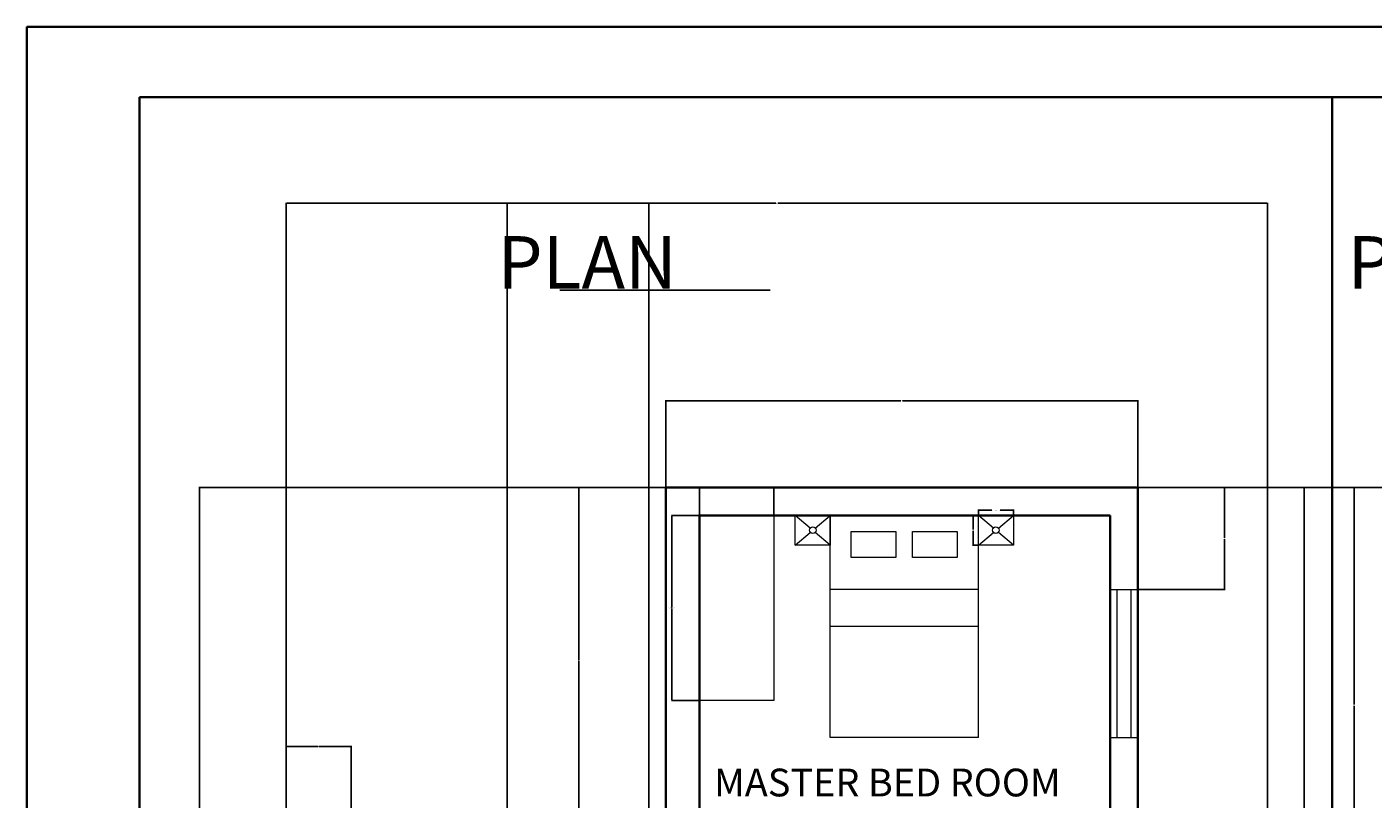
# Model space of a CAD drawing. Units: inches. Extents: x 1762 to 3150, y 1680 to 2382.
# Tile 4 of 6: x 1762 to 2199, y 2132 to 2382. Entities that reach past the tile are written whole.
import ezdxf

# ---------------------------------------------------------------- set-up
doc = ezdxf.new("R2010")
doc.units = ezdxf.units.IN
for name, color, linetype, lineweight in [('A-ANNO-DIMS', 2, 'Continuous', 18), ('A-ANNO-TEXT', 7, 'Continuous', 25), ('A-ANNO-TTLB', 7, 'Continuous', 35), ('A-AREA-IDEN', 7, 'Continuous', 18), ('A-GLAZ', 4, 'Continuous', 18), ('A-WALL', 7, 'Continuous', 35)]:
    doc.layers.add(name, color=color, linetype=linetype, lineweight=lineweight)
doc.layers.add('A-FLOR-CASE', color=242, linetype='Continuous', lineweight=18, true_color=0xcd2027)
doc.layers.add('A-FURN', color=51, linetype='Continuous', lineweight=18, true_color=0xf7f281)
doc.styles.get("Standard").update_dxf_attribs({"font": 'arial.ttf'})
doc.dimstyles.get("Standard").update_dxf_attribs({"dimtxt": 0.18, "dimasz": 0.18, "dimexe": 0.18, "dimexo": 0.0625, "dimgap": 0.09, "dimtad": 0, "dimtih": 1, "dimtoh": 1, "dimdec": 4, "dimzin": 0, "dimdsep": 46, "dimtxsty": 'Standard', "dimcen": 0.09, "dimadec": 0, "dimazin": 0, "dimtfac": 1, "dimtdec": 4, "dimtofl": 0, "dimtmove": 0, "dimatfit": 3, "dimfxl": 1, "dimtolj": 1, "dimtzin": 0, "dimarcsym": 0})

# ---------------------------------------------------------------- blocks, each defined once
blk = doc.blocks.new('WINDOW-48IN')
for p, q in [((0, 48), (9, 48)), ((2.25, 48), (2.25, 0)), ((6.75, 48), (6.75, 0)), ((0, 0), (9, 0))]:
    blk.add_line(p, q)
blk = doc.blocks.new('BED-48X72IN')
for p, q in [((0, 72), (48, 72)), ((0, 72), (0, 0)), ((48, 72), (48, 0)), ((0, 36), (48, 36)), ((0, 24), (48, 24))]:
    blk.add_line(p, q)
for points in [[(6.88, 13.68), (21.36, 13.68), (21.36, 5.23), (6.88, 5.23)], [(26.73, 13.68), (41.21, 13.68), (41.21, 5.23), (26.73, 5.23)]]:
    blk.add_lwpolyline(points, close=True)
blk = doc.blocks.new('NIGHTSTAND')
for p, q in [((0, 9.61), (4.85, 5.5)), ((11.36, 9.61), (6.51, 5.5)), ((4.85, 4.1), (0, 0)), ((6.51, 4.1), (11.36, 0))]:
    blk.add_line(p, q)
blk.add_lwpolyline([(0, 9.61), (11.36, 9.61), (11.36, 0), (0, 0)], close=True)
blk.add_circle((5.68, 4.8), 1.08)
blk = doc.blocks.new('WARDROBE-24X60IN')
for p, q in [((0, 60), (24, 60)), ((24, 60), (24, 0)), ((24, 0), (0, 0))]:
    blk.add_line(p, q)
blk = doc.blocks.new('*D14')
at = {"layer": 'A-ANNO-DIMS', "color": 0, "lineweight": -2, "transparency": 16777216}
for p, q in [((2070.87, 2224.05), (2070.87, 2225.87)), ((2071.05, 2225.69), (2075.18, 2225.69)), ((2082.05, 2225.69), (2077.93, 2225.69)), ((2082.23, 2224.05), (2082.23, 2225.87))]:
    blk.add_line(p, q, dxfattribs=at)
at = {"layer": 'A-ANNO-DIMS', "color": 0, "transparency": 16777216}
for points in [[(2071.05, 2225.72), (2071.05, 2225.66), (2070.87, 2225.69)], [(2082.05, 2225.72), (2082.05, 2225.66), (2082.23, 2225.69)]]:
    blk.add_solid(points, dxfattribs=at)
at = {"layer": 'Defpoints', "color": 0, "transparency": 16777216}
for p in [(2070.87, 2225.69), (2070.87, 2223.99), (2082.23, 2223.99)]:
    blk.add_point(p, dxfattribs=at)
at = {"layer": 'A-ANNO-DIMS', "color": 0, "transparency": 16777216, "insert": (2076.55, 2225.69), "char_height": 0.18, "attachment_point": 5}
blk.add_mtext('\\A1;NIGHTSTAND 11 TYP.', dxfattribs=at)
blk = doc.blocks.new('*D15')
at = {"layer": 'A-ANNO-DIMS', "color": 0, "lineweight": -2, "transparency": 16777216}
for p, q in [((2070.81, 2223.99), (2068.99, 2223.99)), ((2069.17, 2223.81), (2069.17, 2219.37)), ((2069.17, 2214.56), (2069.17, 2219)), ((2070.81, 2214.38), (2068.99, 2214.38))]:
    blk.add_line(p, q, dxfattribs=at)
at = {"layer": 'A-ANNO-DIMS', "color": 0, "transparency": 16777216}
for points in [[(2069.14, 2223.81), (2069.2, 2223.81), (2069.17, 2223.99)], [(2069.14, 2214.56), (2069.2, 2214.56), (2069.17, 2214.38)]]:
    blk.add_solid(points, dxfattribs=at)
at = {"layer": 'Defpoints', "color": 0, "transparency": 16777216}
for p in [(2070.87, 2223.99), (2069.17, 2214.38), (2070.87, 2214.38)]:
    blk.add_point(p, dxfattribs=at)
at = {"layer": 'A-ANNO-DIMS', "color": 0, "transparency": 16777216, "insert": (2069.17, 2219.19), "char_height": 0.18, "attachment_point": 5}
blk.add_mtext('\\A1;10 TYP.', dxfattribs=at)
blk = doc.blocks.new('*D16')
at = {"layer": 'A-ANNO-DIMS', "color": 0, "lineweight": -2, "transparency": 16777216}
for p, q in [((1980.48, 2223.99), (1971.36, 2223.99)), ((1971.54, 2223.81), (1971.54, 2194.17)), ((1971.54, 2164.17), (1971.54, 2193.81)), ((1980.48, 2163.99), (1971.36, 2163.99))]:
    blk.add_line(p, q, dxfattribs=at)
at = {"layer": 'A-ANNO-DIMS', "color": 0, "transparency": 16777216}
for points in [[(1971.51, 2223.81), (1971.57, 2223.81), (1971.54, 2223.99)], [(1971.51, 2164.17), (1971.57, 2164.17), (1971.54, 2163.99)]]:
    blk.add_solid(points, dxfattribs=at)
at = {"layer": 'Defpoints', "color": 0, "transparency": 16777216}
for p in [(1971.54, 2223.99), (1980.54, 2223.99), (1980.54, 2163.99)]:
    blk.add_point(p, dxfattribs=at)
at = {"layer": 'A-ANNO-DIMS', "color": 0, "transparency": 16777216, "insert": (1971.54, 2193.99), "char_height": 0.18, "attachment_point": 5}
blk.add_mtext('\\A1;WARDROBE 60 TYP.', dxfattribs=at)
blk = doc.blocks.new('*D17')
at = {"layer": 'A-ANNO-DIMS', "color": 0, "lineweight": -2, "transparency": 16777216}
for p, q in [((1980.54, 2224.05), (1980.54, 2233.17)), ((1980.72, 2232.99), (1992.01, 2232.99)), ((2004.36, 2232.99), (1993.07, 2232.99)), ((2004.54, 2224.05), (2004.54, 2233.17))]:
    blk.add_line(p, q, dxfattribs=at)
at = {"layer": 'A-ANNO-DIMS', "color": 0, "transparency": 16777216}
for points in [[(1980.72, 2233.02), (1980.72, 2232.96), (1980.54, 2232.99)], [(2004.36, 2233.02), (2004.36, 2232.96), (2004.54, 2232.99)]]:
    blk.add_solid(points, dxfattribs=at)
at = {"layer": 'Defpoints', "color": 0, "transparency": 16777216}
for p in [(2004.54, 2232.99), (1980.54, 2223.99), (2004.54, 2223.99)]:
    blk.add_point(p, dxfattribs=at)
at = {"layer": 'A-ANNO-DIMS', "color": 0, "transparency": 16777216, "insert": (1992.54, 2232.99), "char_height": 0.18, "attachment_point": 5}
blk.add_mtext('\\A1;24 TYP.', dxfattribs=at)
blk = doc.blocks.new('*D32')
at = {"layer": 'A-ANNO-DIMS', "color": 0, "lineweight": -2, "transparency": 16777216}
for p, q in [((1846.54, 2121.05), (1846.54, 2325.32)), ((1846.72, 2325.14), (2005.25, 2325.14)), ((2164.36, 2325.14), (2005.83, 2325.14)), ((2164.54, 2092.05), (2164.54, 2325.32))]:
    blk.add_line(p, q, dxfattribs=at)
at = {"layer": 'A-ANNO-DIMS', "color": 0, "transparency": 16777216}
for points in [[(1846.72, 2325.17), (1846.72, 2325.11), (1846.54, 2325.14)], [(2164.36, 2325.17), (2164.36, 2325.11), (2164.54, 2325.14)]]:
    blk.add_solid(points, dxfattribs=at)
at = {"layer": 'Defpoints', "color": 0, "transparency": 16777216}
for p in [(2164.54, 2325.14), (1846.54, 2120.99), (2164.54, 2091.99)]:
    blk.add_point(p, dxfattribs=at)
at = {"layer": 'A-ANNO-DIMS', "color": 0, "transparency": 16777216, "insert": (2005.54, 2325.14), "char_height": 0.18, "attachment_point": 5}
blk.add_mtext('\\A1;318', dxfattribs=at)
blk = doc.blocks.new('*D33')
at = {"layer": 'A-ANNO-DIMS', "color": 0, "lineweight": -2, "transparency": 16777216}
for p, q in [((1969.475966, 2232.98945), (1818.208466, 2232.98945)), ((1818.388466, 2232.80945), (1818.388466, 1996.16945)), ((1818.388466, 1759.16945), (1818.388466, 1995.80945)), ((1846.475966, 1758.98945), (1818.208466, 1758.98945))]:
    blk.add_line(p, q, dxfattribs=at)
at = {"layer": 'A-ANNO-DIMS', "color": 0, "transparency": 16777216}
for points in [[(1818.358466, 2232.80945), (1818.418466, 2232.80945), (1818.388466, 2232.98945)], [(1818.358466, 1759.16945), (1818.418466, 1759.16945), (1818.388466, 1758.98945)]]:
    blk.add_solid(points, dxfattribs=at)
at = {"layer": 'Defpoints', "color": 0, "transparency": 16777216}
for p in [(1818.388466, 2232.98945), (1969.538466, 2232.98945), (1846.538466, 1758.98945)]:
    blk.add_point(p, dxfattribs=at)
at = {"layer": 'A-ANNO-DIMS', "color": 0, "transparency": 16777216, "insert": (1818.388466, 1995.98945), "char_height": 0.18, "attachment_point": 5}
blk.add_mtext('\\A1;474', dxfattribs=at)
blk = doc.blocks.new('*D34')
at = {"layer": 'A-ANNO-DIMS', "color": 0, "lineweight": -2, "transparency": 16777216}
for p, q in [((1969.54, 2233.05), (1969.54, 2261.32)), ((1969.72, 2261.14), (2045.76, 2261.14)), ((2122.36, 2261.14), (2046.32, 2261.14)), ((2122.54, 2233.05), (2122.54, 2261.32))]:
    blk.add_line(p, q, dxfattribs=at)
at = {"layer": 'A-ANNO-DIMS', "color": 0, "transparency": 16777216}
for points in [[(1969.72, 2261.17), (1969.72, 2261.11), (1969.54, 2261.14)], [(2122.36, 2261.17), (2122.36, 2261.11), (2122.54, 2261.14)]]:
    blk.add_solid(points, dxfattribs=at)
at = {"layer": 'Defpoints', "color": 0, "transparency": 16777216}
for p in [(2122.54, 2261.14), (1969.54, 2232.99), (2122.54, 2232.99)]:
    blk.add_point(p, dxfattribs=at)
at = {"layer": 'A-ANNO-DIMS', "color": 0, "transparency": 16777216, "insert": (2046.04, 2261.14), "char_height": 0.18, "attachment_point": 5}
blk.add_mtext('\\A1;153', dxfattribs=at)
blk = doc.blocks.new('*D38')
at = {"layer": 'A-ANNO-DIMS', "color": 0, "lineweight": -2, "transparency": 16777216}
for p, q in [((2122.6, 2232.99), (2192.87, 2232.99)), ((2192.69, 2232.81), (2192.69, 2162.67)), ((2192.69, 2092.17), (2192.69, 2162.31)), ((2164.6, 2091.99), (2192.87, 2091.99))]:
    blk.add_line(p, q, dxfattribs=at)
at = {"layer": 'A-ANNO-DIMS', "color": 0, "transparency": 16777216}
for points in [[(2192.66, 2232.81), (2192.72, 2232.81), (2192.69, 2232.99)], [(2192.66, 2092.17), (2192.72, 2092.17), (2192.69, 2091.99)]]:
    blk.add_solid(points, dxfattribs=at)
at = {"layer": 'Defpoints', "color": 0, "transparency": 16777216}
for p in [(2122.54, 2232.99), (2192.69, 2232.99), (2164.54, 2091.99)]:
    blk.add_point(p, dxfattribs=at)
at = {"layer": 'A-ANNO-DIMS', "color": 0, "transparency": 16777216, "insert": (2192.69, 2162.49), "char_height": 0.18, "attachment_point": 5}
blk.add_mtext('\\A1;141', dxfattribs=at)
blk = doc.blocks.new('*D44')
at = {"layer": 'A-ANNO-DIMS', "color": 0, "lineweight": -2, "transparency": 16777216}
for p, q in [((1969.48, 2232.99), (1941.21, 2232.99)), ((1941.39, 2232.81), (1941.39, 2177.17)), ((1941.39, 2121.17), (1941.39, 2176.81)), ((1969.48, 2120.99), (1941.21, 2120.99))]:
    blk.add_line(p, q, dxfattribs=at)
at = {"layer": 'A-ANNO-DIMS', "color": 0, "transparency": 16777216}
for points in [[(1941.36, 2232.81), (1941.42, 2232.81), (1941.39, 2232.99)], [(1941.36, 2121.17), (1941.42, 2121.17), (1941.39, 2120.99)]]:
    blk.add_solid(points, dxfattribs=at)
at = {"layer": 'Defpoints', "color": 0, "transparency": 16777216}
for p in [(1941.39, 2232.99), (1969.54, 2232.99), (1969.54, 2120.99)]:
    blk.add_point(p, dxfattribs=at)
at = {"layer": 'A-ANNO-DIMS', "color": 0, "transparency": 16777216, "insert": (1941.39, 2176.99), "char_height": 0.18, "attachment_point": 5}
blk.add_mtext('\\A1;112', dxfattribs=at)
blk = doc.blocks.new('*D45')
at = {"layer": 'A-ANNO-DIMS', "color": 0, "lineweight": -2, "transparency": 16777216}
for p, q in [((1846.54, 2121.05), (1846.54, 2149.32)), ((1846.72, 2149.14), (1856.84, 2149.14)), ((1867.36, 2149.14), (1857.24, 2149.14)), ((1867.54, 2121.05), (1867.54, 2149.32))]:
    blk.add_line(p, q, dxfattribs=at)
at = {"layer": 'A-ANNO-DIMS', "color": 0, "transparency": 16777216}
for points in [[(1846.72, 2149.17), (1846.72, 2149.11), (1846.54, 2149.14)], [(1867.36, 2149.17), (1867.36, 2149.11), (1867.54, 2149.14)]]:
    blk.add_solid(points, dxfattribs=at)
at = {"layer": 'Defpoints', "color": 0, "transparency": 16777216}
for p in [(1867.54, 2149.14), (1846.54, 2120.99), (1867.54, 2120.99)]:
    blk.add_point(p, dxfattribs=at)
at = {"layer": 'A-ANNO-DIMS', "color": 0, "transparency": 16777216, "insert": (1857.04, 2149.14), "char_height": 0.18, "attachment_point": 5}
blk.add_mtext('\\A1;21', dxfattribs=at)
blk = doc.blocks.new('*D46')
at = {"layer": 'A-ANNO-DIMS', "color": 0, "lineweight": -2, "transparency": 16777216}
for p, q in [((2122.6, 2232.99), (2150.87, 2232.99)), ((2150.69, 2232.81), (2150.69, 2216.67)), ((2150.69, 2200.17), (2150.69, 2216.31)), ((2122.6, 2199.99), (2150.87, 2199.99))]:
    blk.add_line(p, q, dxfattribs=at)
at = {"layer": 'A-ANNO-DIMS', "color": 0, "transparency": 16777216}
for points in [[(2150.66, 2232.81), (2150.72, 2232.81), (2150.69, 2232.99)], [(2150.66, 2200.17), (2150.72, 2200.17), (2150.69, 2199.99)]]:
    blk.add_solid(points, dxfattribs=at)
at = {"layer": 'Defpoints', "color": 0, "transparency": 16777216}
for p in [(2122.54, 2232.99), (2122.54, 2199.99), (2150.69, 2199.99)]:
    blk.add_point(p, dxfattribs=at)
at = {"layer": 'A-ANNO-DIMS', "color": 0, "transparency": 16777216, "insert": (2150.69, 2216.49), "char_height": 0.18, "attachment_point": 5}
blk.add_mtext('\\A1;33', dxfattribs=at)
blk = doc.blocks.new('*D57')
at = {"layer": 'A-ANNO-DIMS', "color": 0, "lineweight": -2, "transparency": 16777216}
for p, q in [((1918.11, 1951.12), (1918.11, 2325.32)), ((1918.29, 2325.14), (1940.7, 2325.14)), ((1963.91, 2325.14), (1941.5, 2325.14)), ((1964.09, 1951.12), (1964.09, 2325.32))]:
    blk.add_line(p, q, dxfattribs=at)
at = {"layer": 'A-ANNO-DIMS', "color": 0, "transparency": 16777216}
for points in [[(1918.29, 2325.17), (1918.29, 2325.11), (1918.11, 2325.14)], [(1963.91, 2325.17), (1963.91, 2325.11), (1964.09, 2325.14)]]:
    blk.add_solid(points, dxfattribs=at)
at = {"layer": 'Defpoints', "color": 0, "transparency": 16777216}
for p in [(1964.09, 2325.14), (1918.11, 1951.05), (1964.09, 1951.05)]:
    blk.add_point(p, dxfattribs=at)
at = {"layer": 'A-ANNO-DIMS', "color": 0, "transparency": 16777216, "insert": (1941.1, 2325.14), "char_height": 0.18, "attachment_point": 5}
blk.add_mtext('\\A1;45.97', dxfattribs=at)
blk = doc.blocks.new('*D65')
at = {"layer": 'A-ANNO-DIMS', "color": 0, "lineweight": -2, "transparency": 16777216}
for p, q in [((2364.876105, 2232.98945), (2176.268936, 2232.98945)), ((2176.448936, 2232.80945), (2176.448936, 1996.16945)), ((2176.448936, 1759.16945), (2176.448936, 1995.80945)), ((2239.876105, 1758.98945), (2176.268936, 1758.98945))]:
    blk.add_line(p, q, dxfattribs=at)
at = {"layer": 'A-ANNO-DIMS', "color": 0, "transparency": 16777216}
for points in [[(2176.418936, 2232.80945), (2176.478936, 2232.80945), (2176.448936, 2232.98945)], [(2176.418936, 1759.16945), (2176.478936, 1759.16945), (2176.448936, 1758.98945)]]:
    blk.add_solid(points, dxfattribs=at)
at = {"layer": 'Defpoints', "color": 0, "transparency": 16777216}
for p in [(2176.448936, 2232.98945), (2364.938605, 2232.98945), (2239.938605, 1758.98945)]:
    blk.add_point(p, dxfattribs=at)
at = {"layer": 'A-ANNO-DIMS', "color": 0, "transparency": 16777216, "insert": (2176.448936, 1995.98945), "char_height": 0.18, "attachment_point": 5}
blk.add_mtext('\\A1;474', dxfattribs=at)

msp = doc.modelspace()

# ---------------------------------------------------------------- linework, layer by layer
at = {"layer": 'A-ANNO-TEXT'}
msp.add_line((1935.1794, 2296.9856), (2003.4226, 2296.9856), dxfattribs=at)
at = {"layer": 'A-ANNO-TTLB'}
msp.add_line((2185.5413, 2359.5805), (2185.5413, 1709.6712), dxfattribs=at)
for points in [[(1762.4998, 2382.3025), (3150.3176, 2382.3025), (3150.3176, 1679.5742), (1762.4998, 1679.5742)], [(1799.0337, 2359.5805), (3111.4319, 2359.5805), (3111.4319, 1709.6712), (1799.0337, 1709.6712)]]:
    msp.add_lwpolyline(points, close=True, dxfattribs=at)
at = {"layer": 'A-WALL'}
for p, q in [((1969.5385, 2232.9895), (2122.5385, 2232.9895)), ((1969.5385, 2232.9895), (1969.5385, 2120.9895)), ((2122.5385, 2232.9895), (2122.5385, 2091.9895)), ((1980.5385, 2223.9895), (1980.5385, 2091.9895)), ((1980.5385, 2223.9895), (2113.5385, 2223.9895)), ((2113.5385, 2223.9895), (2113.5385, 2091.9895))]:
    msp.add_line(p, q, dxfattribs=at)

# ---------------------------------------------------------------- block references
at = {"layer": 'A-FLOR-CASE'}
msp.add_blockref('WARDROBE-24X60IN', (1980.538, 2163.989), dxfattribs=at)
at = {"layer": 'A-FURN', "rotation": 180}
for name, p in [('NIGHTSTAND', (2022.8745, 2223.9899)), ('BED-48X72IN', (2070.8746, 2223.9899)), ('NIGHTSTAND', (2082.2316, 2223.9899))]:
    msp.add_blockref(name, p, dxfattribs=at)
at = {"layer": 'A-GLAZ'}
msp.add_blockref('WINDOW-48IN', (2113.538, 2151.989), dxfattribs=at)

# ---------------------------------------------------------------- texts
at = {"layer": 'A-ANNO-TEXT'}
for s, p in [('               PLAN', (1837.0529, 2297.5007)), ('            PLINTH AND SLAB BEAM LAYOUT', (2128.1301, 2297.5007))]:
    msp.add_text(s, height=17, dxfattribs=at).set_placement(p)
at = {"layer": 'A-AREA-IDEN'}
msp.add_text(' MASTER BED ROOM', height=9, dxfattribs=at).set_placement((1982.4401, 2132.9128))

# ---------------------------------------------------------------- dimensions: what is measured, and where the dimension line sits
at = {"layer": 'A-ANNO-DIMS'}
for base, p1, p2, override, picture, middle in [((2164.5385, 2325.1356), (1846.5385, 2120.9895), (2164.5385, 2091.9895), {"dimdec": 0, "dimlfac": 1, "dimrnd": 0, "dimzin": 0, "dimdsep": 46, "dimlunit": 2}, '*D32', (2005.5385, 2325.1356)), ((1964.0853, 2325.1356), (1918.1134, 1951.0543), (1964.0853, 1951.0543), {"dimdec": 2, "dimlfac": 1, "dimrnd": 0, "dimzin": 0, "dimdsep": 46, "dimlunit": 2}, '*D57', (1941.0994, 2325.1356)), ((2122.5385, 2261.1395), (1969.5385, 2232.9895), (2122.5385, 2232.9895), {"dimdec": 0, "dimlfac": 1, "dimrnd": 0, "dimzin": 0, "dimdsep": 46, "dimlunit": 2}, '*D34', (2046.0385, 2261.1395)), ((1867.5385, 2149.1395), (1846.5385, 2120.9895), (1867.5385, 2120.9895), {"dimdec": 0, "dimlfac": 1, "dimrnd": 0, "dimzin": 0, "dimdsep": 46, "dimlunit": 2}, '*D45', (1857.0385, 2149.1395))]:
    dim = msp.add_linear_dim(base=base, p1=p1, p2=p2, dimstyle='Standard', override=override, dxfattribs=at)
    dim.commit()
    dim.dimension.update_dxf_attribs({"geometry": picture, "text_midpoint": middle})
for base, p1, p2, angle, picture, middle in [((1818.3885, 2232.9895), (1846.5385, 1758.9895), (1969.5385, 2232.9895), 90, '*D33', (1818.3885, 1995.9895)), ((1941.3885, 2232.9895), (1969.5385, 2120.9895), (1969.5385, 2232.9895), 90, '*D44', (1941.3885, 2176.9895)), ((2192.6885, 2232.9895), (2164.5385, 2091.9895), (2122.5385, 2232.9895), 90, '*D38', (2192.6885, 2162.4895)), ((2150.6885, 2199.9895), (2122.5385, 2232.9895), (2122.5385, 2199.9895), 270, '*D46', (2150.6885, 2216.4895)), ((2176.4489, 2232.9895), (2239.9386, 1758.9895), (2364.9386, 2232.9895), 90, '*D65', (2176.4489, 1995.9894))]:
    dim = msp.add_linear_dim(base=base, p1=p1, p2=p2, angle=angle, dimstyle='Standard', override={"dimdec": 0, "dimlfac": 1, "dimrnd": 0, "dimzin": 0, "dimdsep": 46, "dimlunit": 2}, dxfattribs=at)
    dim.commit()
    dim.dimension.update_dxf_attribs({"geometry": picture, "text_midpoint": middle})
dim = msp.add_linear_dim(base=(2004.5385, 2232.9895), p1=(1980.5385, 2223.9895), p2=(2004.5385, 2223.9895), text='<> TYP.', dimstyle='Standard', override={"dimdec": 0, "dimlfac": 1, "dimrnd": 0, "dimzin": 0, "dimdsep": 46, "dimlunit": 2}, dxfattribs=at)
dim.commit()
dim.dimension.update_dxf_attribs({"geometry": '*D17', "text_midpoint": (1992.5385, 2232.9895)})
for base, p1, p2, angle, text, picture, middle in [((2070.8742, 2225.693), (2082.2313, 2223.9895), (2070.8742, 2223.9895), 180, 'NIGHTSTAND <> TYP.', '*D14', (2076.5527, 2225.693)), ((1971.5385, 2223.9895), (1980.5385, 2163.9895), (1980.5385, 2223.9895), 90, 'WARDROBE <> TYP.', '*D16', (1971.5385, 2193.9895)), ((2069.1706, 2214.3832), (2070.8742, 2223.9895), (2070.8742, 2214.3832), 270, '<> TYP.', '*D15', (2069.1706, 2219.1863))]:
    dim = msp.add_linear_dim(base=base, p1=p1, p2=p2, angle=angle, text=text, dimstyle='Standard', override={"dimdec": 0, "dimlfac": 1, "dimrnd": 0, "dimzin": 0, "dimdsep": 46, "dimlunit": 2}, dxfattribs=at)
    dim.commit()
    dim.dimension.update_dxf_attribs({"geometry": picture, "text_midpoint": middle})

doc.saveas('drawing.dxf')
